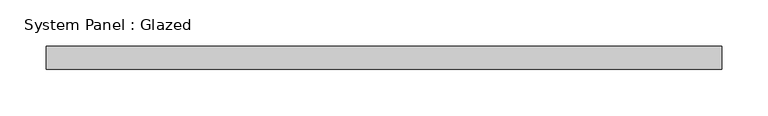
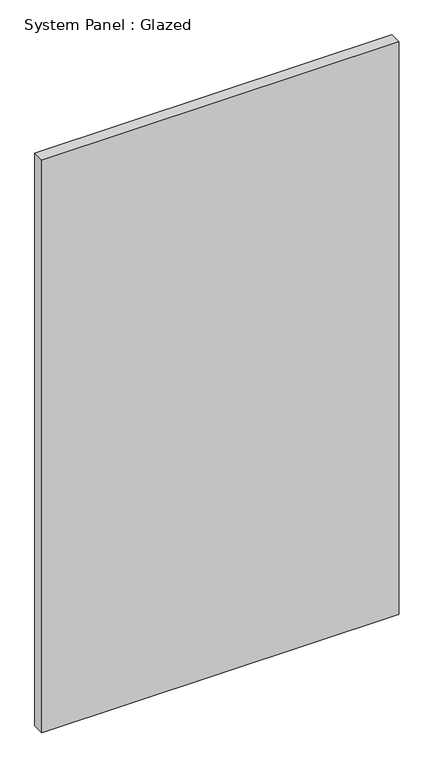
"""IFC4 building model written with IfcOpenShell, lengths in millimetres: plate geometry, System Panel : Glazed."""

from ifc_helpers import new_model, si_unit, origin, origin_with_axes, place, context, project, spatial, polyline, outline, extrude, source, transform, mapped, element, save


def system_panel_glazed_b614e8ed(model_context):
    return source(origin(), model_context, "Body", "SweptSolid", [
        extrude(outline(polyline([(365.0, 24.5), (-365.0, 24.5), (-365.0, 49.5), (365.0, 49.5), (365.0, 24.5)])), origin_with_axes(), (0.0, 0.0, 1.0), 1237.5),
    ])


if __name__ == "__main__":
    model = new_model("IFC4")
    model_context = context("Model", 3, world=origin())
    ifc_project = project(units=[si_unit("LENGTHUNIT", "METRE", prefix="MILLI")], contexts=[model_context])
    site = spatial("IfcSite", under=ifc_project)
    building = spatial("IfcBuilding", under=site)
    placement = place(None, origin())
    system_panel_glazed_shape = system_panel_glazed_b614e8ed(model_context)
    element("IfcPlate", 1, ObjectType="System Panel : Glazed", at=placement, inside=building, context=model_context, shape_type="MappedRepresentation", body=[
        mapped(system_panel_glazed_shape, transform((0.0, 0.0, 0.0), x_axis=(1.0, 0.0, 0.0), y_axis=(0.0, 1.0, 0.0), z_axis=(0.0, 0.0, 1.0))),
    ])
    save(model, "model.ifc")

# Revit data of these elements
# Element 1 (IfcPlate, "System Panel : Glazed")
#   Materials on its faces: "Glass"
# Materials
#   "Glass": class "Glass", colour RGB 218 227 224, transparency 0.85, Description = "Soda Lime Glass", Cost = 0
